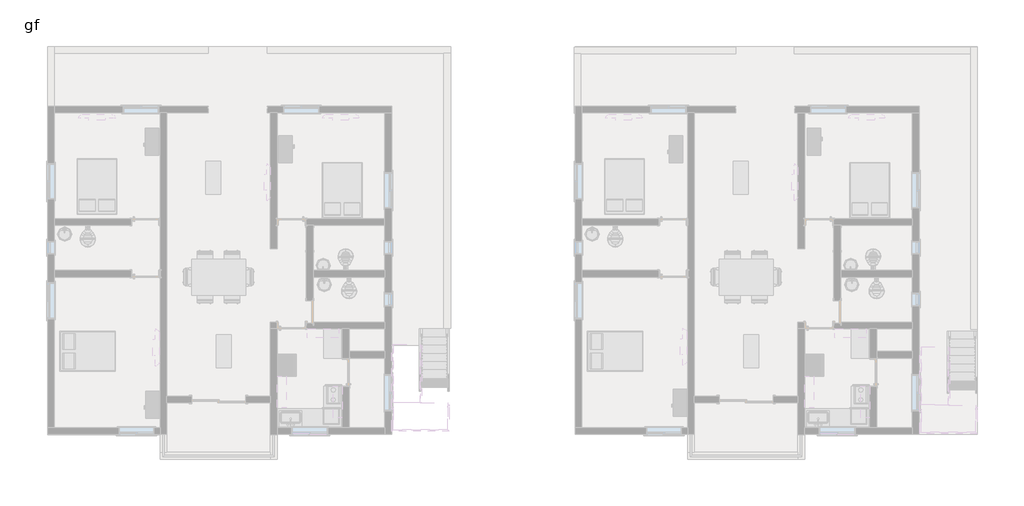
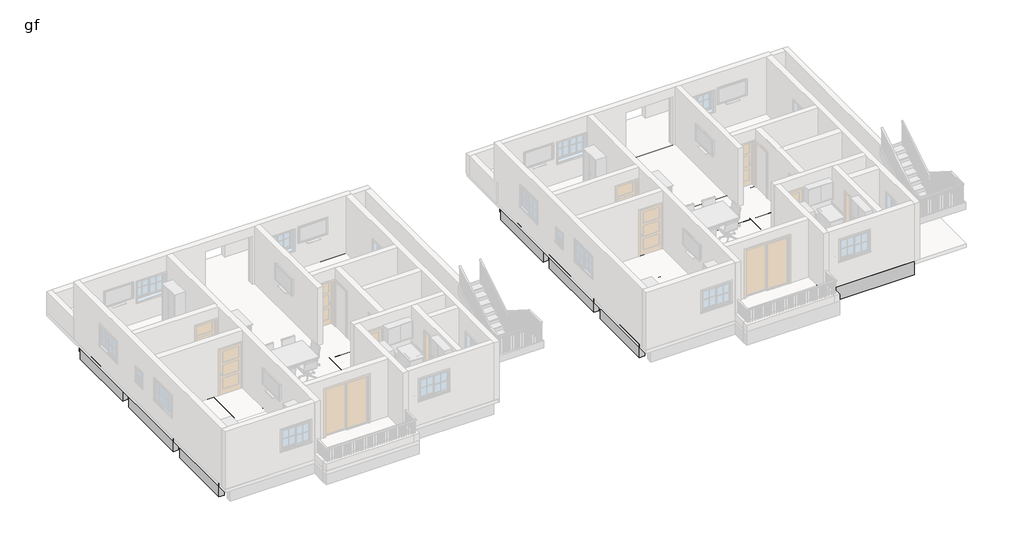
# One storey, part 3 of 8: 32 beams.
"""IFC4 building model written with IfcOpenShell, lengths in millimetres."""

from ifc_helpers import new_model, si_unit, origin, origin_with_axes, place, context, project, spatial, polyline, outline, extrude, faceted_brep, element, save

model = new_model("IFC4")

# Units and contexts
model_context = context("Model", 3, world=origin())
ifc_project = project(units=[si_unit("LENGTHUNIT", "METRE", prefix="MILLI")], contexts=[model_context])

# Site, building, storey
site = spatial("IfcSite", under=ifc_project)
building = spatial("IfcBuilding", under=site)
storey = spatial("IfcBuildingStorey", under=building, Name="gf", Elevation=609.6)

# Beams
placement = place(None, origin())
element("IfcBeam", 1, ObjectType="Concrete-Rectangular Beam", at=placement, inside=storey, context=model_context, shape_type="Brep", body=[
    faceted_brep([(-16071.9993763, -1252.5064015, 609.6), (-16300.5993763, -1252.5064015, 609.6), (-16300.5993763, -4148.1064015, 609.6), (-16071.9993763, -4148.1064015, 609.6), (-16300.5993763, -1252.5064015, 0.0), (-16300.5993763, -4148.1064015, 0.0), (-16071.9993763, -1252.5064015, 0.0), (-16071.9993763, -4148.1064015, 0.0)], [[[0, 1, 2, 3]], [[1, 4, 5, 2]], [[4, 6, 7, 5]], [[6, 0, 3, 7]], [[1, 0, 6, 4]], [[3, 2, 5, 7]]]),
    faceted_brep([(-16300.5993763, 6062.6935985, 609.6), (-16071.9993763, 6062.6935985, 609.6), (-16071.9993763, 6062.6935985, 0.0), (-16300.5993763, 6062.6935985, 0.0), (-16071.9993763, 2938.4935985, 609.6), (-16300.5993763, 2938.4935985, 609.6), (-16300.5993763, 2938.4935985, 0.0), (-16071.9993763, 2938.4935985, 0.0)], [[[0, 1, 2, 3]], [[4, 5, 6, 7]], [[1, 0, 5, 4]], [[0, 3, 6, 5]], [[3, 2, 7, 6]], [[2, 1, 4, 7]]]),
    faceted_brep([(-16300.5993763, 2481.2935985, 609.6), (-16071.9993763, 2481.2935985, 609.6), (-16071.9993763, 2481.2935985, 0.0), (-16300.5993763, 2481.2935985, 0.0), (-16071.9993763, -795.3064015, 609.6), (-16300.5993763, -795.3064015, 609.6), (-16300.5993763, -795.3064015, 0.0), (-16071.9993763, -795.3064015, 0.0), (-16071.9993763, 728.6935985, 609.6), (-16071.9993763, 957.2935985, 609.6), (-16071.9993763, 957.2935985, 0.0), (-16071.9993763, 728.6935985, 0.0)], [[[0, 1, 2, 3]], [[4, 5, 6, 7]], [[1, 0, 5, 4, 8, 9]], [[0, 3, 6, 5]], [[3, 2, 10, 11, 7, 6]], [[2, 1, 9, 8, 4, 7, 11, 10]]]),
])
element("IfcBeam", 2, ObjectType="Concrete-Rectangular Beam", at=placement, inside=storey, context=model_context, shape_type="SweptSolid", body=[
    extrude(outline(polyline([(-16071.9993763, 6291.2935985), (-16071.9993763, 6519.8935985), (-12490.5993763, 6519.8935985), (-12490.5993763, 6291.2935985), (-16071.9993763, 6291.2935985)])), origin_with_axes(), (0.0, 0.0, 1.0), 609.6),
    extrude(outline(polyline([(-12261.9993763, 6291.2935985), (-12261.9993763, 6519.8935985), (-8756.7993763, 6519.8935985), (-8756.7993763, 6291.2935985), (-12261.9993763, 6291.2935985)])), origin_with_axes(), (0.0, 0.0, 1.0), 609.6),
    extrude(outline(polyline([(-8528.1993763, 6291.2935985), (-8528.1993763, 6519.8935985), (-4870.5993763, 6519.8935985), (-4870.5993763, 6291.2935985), (-8528.1993763, 6291.2935985)])), origin_with_axes(), (0.0, 0.0, 1.0), 609.6),
])
element("IfcBeam", 3, ObjectType="Concrete-Rectangular Beam", at=placement, inside=storey, context=model_context, shape_type="Brep", body=[
    faceted_brep([(-12261.9993763, -1252.5064015, 609.6), (-12490.5993763, -1252.5064015, 609.6), (-12490.5993763, -4148.1064015, 609.6), (-12261.9993763, -4148.1064015, 609.6), (-12261.9993763, -3538.5064015, 609.6), (-12261.9993763, -3309.9064015, 609.6), (-12490.5993763, -1252.5064015, 0.0), (-12490.5993763, -4148.1064015, 0.0), (-12261.9993763, -1252.5064015, 0.0), (-12261.9993763, -3309.9064015, 0.0), (-12261.9993763, -3538.5064015, 0.0), (-12261.9993763, -4148.1064015, 0.0)], [[[0, 1, 2, 3, 4, 5]], [[1, 6, 7, 2]], [[6, 8, 9, 10, 11, 7]], [[8, 0, 5, 4, 3, 11, 10, 9]], [[1, 0, 8, 6]], [[3, 2, 7, 11]]]),
    faceted_brep([(-12490.5993763, 6062.6935985, 609.6), (-12261.9993763, 6062.6935985, 609.6), (-12261.9993763, 6062.6935985, 0.0), (-12490.5993763, 6062.6935985, 0.0), (-12261.9993763, 2938.4935985, 609.6), (-12490.5993763, 2938.4935985, 609.6), (-12490.5993763, 2938.4935985, 0.0), (-12261.9993763, 2938.4935985, 0.0)], [[[0, 1, 2, 3]], [[4, 5, 6, 7]], [[1, 0, 5, 4]], [[0, 3, 6, 5]], [[3, 2, 7, 6]], [[2, 1, 4, 7]]]),
    faceted_brep([(-12490.5993763, 2481.2935985, 609.6), (-12261.9993763, 2481.2935985, 609.6), (-12261.9993763, 2481.2935985, 0.0), (-12490.5993763, 2481.2935985, 0.0), (-12261.9993763, -795.3064015, 609.6), (-12490.5993763, -795.3064015, 609.6), (-12490.5993763, -795.3064015, 0.0), (-12261.9993763, -795.3064015, 0.0), (-12490.5993763, 957.2935985, 609.6), (-12490.5993763, 728.6935985, 609.6), (-12261.9993763, 728.6935985, 609.6), (-12261.9993763, 957.2935985, 609.6), (-12490.5993763, 957.2935985, 0.0), (-12490.5993763, 728.6935985, 0.0), (-12261.9993763, 957.2935985, 0.0), (-12261.9993763, 728.6935985, 0.0)], [[[0, 1, 2, 3]], [[4, 5, 6, 7]], [[1, 0, 8, 9, 5, 4, 10, 11]], [[0, 3, 12, 13, 6, 5, 9, 8]], [[3, 2, 14, 15, 7, 6, 13, 12]], [[2, 1, 11, 10, 4, 7, 15, 14]]]),
])
element("IfcBeam", 4, ObjectType="Concrete-Rectangular Beam", at=placement, inside=storey, context=model_context, shape_type="Brep", body=[
    faceted_brep([(-8528.1993763, 6062.6935985, 609.6), (-8756.7993763, 6062.6935985, 609.6), (-8756.7993763, 2938.4935985, 609.6), (-8528.1993763, 2938.4935985, 609.6), (-8528.1993763, 6062.6935985, 0.0), (-8528.1993763, 2938.4935985, 0.0), (-8756.7993763, 6062.6935985, 0.0), (-8756.7993763, 2938.4935985, 0.0)], [[[0, 1, 2, 3]], [[4, 0, 3, 5]], [[6, 4, 5, 7]], [[1, 6, 7, 2]], [[1, 0, 4, 6]], [[3, 2, 7, 5]]]),
    faceted_brep([(-8528.1993763, -5214.9064015, 609.6), (-8756.7993763, -5214.9064015, 609.6), (-8756.7993763, -5214.9064015, 0.0), (-8528.1993763, -5214.9064015, 0.0), (-8756.7993763, -4605.3064015, 609.6), (-8528.1993763, -4605.3064015, 609.6), (-8528.1993763, -4605.3064015, 0.0), (-8756.7993763, -4605.3064015, 0.0)], [[[0, 1, 2, 3]], [[4, 5, 6, 7]], [[1, 0, 5, 4]], [[0, 3, 6, 5]], [[3, 2, 7, 6]], [[2, 1, 4, 7]]]),
    faceted_brep([(-8528.1993763, -4148.1064015, 609.6), (-8756.7993763, -4148.1064015, 609.6), (-8756.7993763, -4148.1064015, 0.0), (-8528.1993763, -4148.1064015, 0.0), (-8756.7993763, -1252.5064015, 609.6), (-8528.1993763, -1252.5064015, 609.6), (-8528.1993763, -1252.5064015, 0.0), (-8756.7993763, -1252.5064015, 0.0), (-8756.7993763, -3309.9064015, 609.6), (-8756.7993763, -3538.5064015, 609.6), (-8756.7993763, -3538.5064015, 0.0), (-8756.7993763, -3309.9064015, 0.0)], [[[0, 1, 2, 3]], [[4, 5, 6, 7]], [[1, 0, 5, 4, 8, 9]], [[0, 3, 6, 5]], [[3, 2, 10, 11, 7, 6]], [[2, 1, 9, 8, 4, 7, 11, 10]]]),
    faceted_brep([(-8756.7993763, 2481.2935985, 609.6), (-8528.1993763, 2481.2935985, 609.6), (-8528.1993763, 2481.2935985, 0.0), (-8756.7993763, 2481.2935985, 0.0), (-8528.1993763, -795.3064015, 609.6), (-8756.7993763, -795.3064015, 609.6), (-8756.7993763, -795.3064015, 0.0), (-8528.1993763, -795.3064015, 0.0), (-8756.7993763, 957.2935985, 609.6), (-8756.7993763, 728.6935985, 609.6), (-8528.1993763, 728.6935985, 609.6), (-8528.1993763, 957.2935985, 609.6), (-8528.1993763, 728.6935985, 0.0), (-8528.1993763, 957.2935985, 0.0), (-8756.7993763, 728.6935985, 0.0), (-8756.7993763, 957.2935985, 0.0)], [[[0, 1, 2, 3]], [[4, 5, 6, 7]], [[1, 0, 8, 9, 5, 4, 10, 11]], [[2, 1, 11, 10, 4, 7, 12, 13]], [[3, 2, 13, 12, 7, 6, 14, 15]], [[0, 3, 15, 14, 6, 5, 9, 8]]]),
])
element("IfcBeam", 5, ObjectType="Concrete-Rectangular Beam", at=placement, inside=storey, context=model_context, shape_type="Brep", body=[
    faceted_brep([(-4641.9993763, -1023.9064015, 609.6), (-4870.5993763, -1023.9064015, 609.6), (-4870.5993763, -1785.9064015, 609.6), (-4870.5993763, -2014.5064015, 609.6), (-4870.5993763, -4148.1064015, 609.6), (-4641.9993763, -4148.1064015, 609.6), (-4870.5993763, -1023.9064015, 0.0), (-4870.5993763, -1785.9064015, 0.0), (-4870.5993763, -2014.5064015, 0.0), (-4870.5993763, -4148.1064015, 0.0), (-4641.9993763, -1023.9064015, 0.0), (-4641.9993763, -4148.1064015, 0.0)], [[[0, 1, 2, 3, 4, 5]], [[1, 6, 7, 8, 9, 4, 3, 2]], [[6, 10, 11, 9, 8, 7]], [[10, 0, 5, 11]], [[1, 0, 10, 6]], [[5, 4, 9, 11]]]),
    faceted_brep([(-4870.5993763, 6062.6935985, 609.6), (-4641.9993763, 6062.6935985, 609.6), (-4641.9993763, 6062.6935985, 0.0), (-4870.5993763, 6062.6935985, 0.0), (-4641.9993763, 2938.4935985, 609.6), (-4870.5993763, 2938.4935985, 609.6), (-4870.5993763, 2938.4935985, 0.0), (-4641.9993763, 2938.4935985, 0.0)], [[[0, 1, 2, 3]], [[4, 5, 6, 7]], [[1, 0, 5, 4]], [[0, 3, 6, 5]], [[3, 2, 7, 6]], [[2, 1, 4, 7]]]),
    faceted_brep([(-4870.5993763, 2481.2935985, 609.6), (-4641.9993763, 2481.2935985, 609.6), (-4641.9993763, 2481.2935985, 0.0), (-4870.5993763, 2481.2935985, 0.0), (-4641.9993763, -566.7064015, 609.6), (-4870.5993763, -566.7064015, 609.6), (-4870.5993763, -566.7064015, 0.0), (-4641.9993763, -566.7064015, 0.0), (-4870.5993763, 957.2935985, 609.6), (-4870.5993763, 728.6935985, 609.6), (-4870.5993763, 957.2935985, 0.0), (-4870.5993763, 728.6935985, 0.0)], [[[0, 1, 2, 3]], [[4, 5, 6, 7]], [[1, 0, 8, 9, 5, 4]], [[0, 3, 10, 11, 6, 5, 9, 8]], [[3, 2, 7, 6, 11, 10]], [[2, 1, 4, 7]]]),
])
element("IfcBeam", 6, ObjectType="Concrete-Rectangular Beam", at=placement, inside=storey, context=model_context, shape_type="Brep", body=[
    faceted_brep([(-7308.9993763, 2709.8935985, 609.6), (-7537.5993763, 2709.8935985, 609.6), (-7537.5993763, 2481.2935985, 609.6), (-7537.5993763, 957.2935985, 609.6), (-7537.5993763, 728.6935985, 609.6), (-7537.5993763, -795.3064015, 609.6), (-7308.9993763, -795.3064015, 609.6), (-7308.9993763, 728.6935985, 609.6), (-7308.9993763, 957.2935985, 609.6), (-7308.9993763, 2481.2935985, 609.6), (-7308.9993763, 2709.8935985, 0.0), (-7308.9993763, -795.3064015, 0.0), (-7308.9993763, 728.6935985, 0.0), (-7308.9993763, 957.2935985, 0.0), (-7308.9993763, 2481.2935985, 0.0), (-7537.5993763, 2709.8935985, 0.0), (-7537.5993763, -795.3064015, 0.0), (-7537.5993763, 728.6935985, 0.0), (-7537.5993763, 957.2935985, 0.0), (-7537.5993763, 2481.2935985, 0.0)], [[[0, 1, 2, 3, 4, 5, 6, 7, 8, 9]], [[10, 0, 9, 8, 7, 6, 11, 12, 13, 14]], [[15, 10, 14, 13, 12, 11, 16, 17, 18, 19]], [[1, 15, 19, 18, 17, 16, 5, 4, 3, 2]], [[6, 5, 16, 11]], [[1, 0, 10, 15]]]),
])
element("IfcBeam", 7, ObjectType="Concrete-Rectangular Beam", at=placement, inside=storey, context=model_context, shape_type="SweptSolid", body=[
    extrude(outline(polyline([(-7308.9993763, 2481.2935985), (-7308.9993763, 2709.8935985), (-4870.5993763, 2709.8935985), (-4870.5993763, 2481.2935985), (-7308.9993763, 2481.2935985)])), origin_with_axes(), (0.0, 0.0, 1.0), 609.6),
])
element("IfcBeam", 8, ObjectType="Concrete-Rectangular Beam", at=placement, inside=storey, context=model_context, shape_type="SweptSolid", body=[
    extrude(outline(polyline([(-4870.5993763, 957.2935985), (-4870.5993763, 728.6935985), (-7308.9993763, 728.6935985), (-7308.9993763, 957.2935985), (-4870.5993763, 957.2935985)])), origin_with_axes(), (0.0, 0.0, 1.0), 609.6),
])
element("IfcBeam", 9, ObjectType="Concrete-Rectangular Beam", at=placement, inside=storey, context=model_context, shape_type="SweptSolid", body=[
    extrude(outline(polyline([(-12261.9993763, 2481.2935985), (-12261.9993763, 2709.8935985), (-8756.7993763, 2709.8935985), (-8756.7993763, 2481.2935985), (-12261.9993763, 2481.2935985)])), origin_with_axes(), (0.0, 0.0, 1.0), 609.6),
    extrude(outline(polyline([(-7537.5993763, 2709.8935985), (-7537.5993763, 2481.2935985), (-8528.1993763, 2481.2935985), (-8528.1993763, 2709.8935985), (-7537.5993763, 2709.8935985)])), origin_with_axes(), (0.0, 0.0, 1.0), 609.6),
])
element("IfcBeam", 10, ObjectType="Concrete-Rectangular Beam", at=placement, inside=storey, context=model_context, shape_type="Brep", body=[
    faceted_brep([(-13481.1993763, 2709.8935985, 609.6), (-13709.7993763, 2709.8935985, 609.6), (-13709.7993763, 957.2935985, 609.6), (-13709.7993763, 728.6935985, 609.6), (-13709.7993763, -795.3064015, 609.6), (-13481.1993763, -795.3064015, 609.6), (-13481.1993763, 728.6935985, 609.6), (-13481.1993763, 957.2935985, 609.6), (-13481.1993763, 2481.2935985, 609.6), (-13709.7993763, 2709.8935985, 0.0), (-13709.7993763, 957.2935985, 0.0), (-13709.7993763, 728.6935985, 0.0), (-13709.7993763, -795.3064015, 0.0), (-13481.1993763, 2709.8935985, 0.0), (-13481.1993763, 2481.2935985, 0.0), (-13481.1993763, 957.2935985, 0.0), (-13481.1993763, 728.6935985, 0.0), (-13481.1993763, -795.3064015, 0.0)], [[[0, 1, 2, 3, 4, 5, 6, 7, 8]], [[1, 9, 10, 11, 12, 4, 3, 2]], [[9, 13, 14, 15, 16, 17, 12, 11, 10]], [[13, 0, 8, 7, 6, 5, 17, 16, 15, 14]], [[5, 4, 12, 17]], [[1, 0, 13, 9]]]),
])
element("IfcBeam", 11, ObjectType="Concrete-Rectangular Beam", at=placement, inside=storey, context=model_context, shape_type="SweptSolid", body=[
    extrude(outline(polyline([(-16071.9993763, 728.6935985), (-16071.9993763, 957.2935985), (-13709.7993763, 957.2935985), (-13709.7993763, 728.6935985), (-16071.9993763, 728.6935985)])), origin_with_axes(), (0.0, 0.0, 1.0), 609.6),
])
element("IfcBeam", 12, ObjectType="Concrete-Rectangular Beam", at=placement, inside=storey, context=model_context, shape_type="SweptSolid", body=[
    extrude(outline(polyline([(-12490.5993763, 957.2935985), (-12490.5993763, 728.6935985), (-13481.1993763, 728.6935985), (-13481.1993763, 957.2935985), (-12490.5993763, 957.2935985)])), origin_with_axes(), (0.0, 0.0, 1.0), 609.6),
])
element("IfcBeam", 13, ObjectType="Concrete-Rectangular Beam", at=placement, inside=storey, context=model_context, shape_type="SweptSolid", body=[
    extrude(outline(polyline([(-12261.9993763, 728.6935985), (-12261.9993763, 957.2935985), (-8756.7993763, 957.2935985), (-8756.7993763, 728.6935985), (-12261.9993763, 728.6935985)])), origin_with_axes(), (0.0, 0.0, 1.0), 609.6),
    extrude(outline(polyline([(-7537.5993763, 957.2935985), (-7537.5993763, 728.6935985), (-8528.1993763, 728.6935985), (-8528.1993763, 957.2935985), (-7537.5993763, 957.2935985)])), origin_with_axes(), (0.0, 0.0, 1.0), 609.6),
])
element("IfcBeam", 14, ObjectType="Concrete-Rectangular Beam", at=placement, inside=storey, context=model_context, shape_type="SweptSolid", body=[
    extrude(outline(polyline([(-12490.5993763, 2709.8935985), (-12490.5993763, 2481.2935985), (-13481.1993763, 2481.2935985), (-13481.1993763, 2709.8935985), (-12490.5993763, 2709.8935985)])), origin_with_axes(), (0.0, 0.0, 1.0), 609.6),
])
element("IfcBeam", 15, ObjectType="Concrete-Rectangular Beam", at=placement, inside=storey, context=model_context, shape_type="Brep", body=[
    faceted_brep([(1802.5761273, -1252.5064015, 609.6), (1573.9761273, -1252.5064015, 609.6), (1573.9761273, -4148.1064015, 609.6), (1802.5761273, -4148.1064015, 609.6), (1573.9761273, -1252.5064015, 0.0), (1573.9761273, -4148.1064015, 0.0), (1802.5761273, -1252.5064015, 0.0), (1802.5761273, -4148.1064015, 0.0)], [[[0, 1, 2, 3]], [[1, 4, 5, 2]], [[4, 6, 7, 5]], [[6, 0, 3, 7]], [[1, 0, 6, 4]], [[3, 2, 5, 7]]]),
    faceted_brep([(1573.9761273, 6062.6935985, 609.6), (1802.5761273, 6062.6935985, 609.6), (1802.5761273, 6062.6935985, 0.0), (1573.9761273, 6062.6935985, 0.0), (1802.5761273, 2938.4935985, 609.6), (1573.9761273, 2938.4935985, 609.6), (1573.9761273, 2938.4935985, 0.0), (1802.5761273, 2938.4935985, 0.0)], [[[0, 1, 2, 3]], [[4, 5, 6, 7]], [[1, 0, 5, 4]], [[0, 3, 6, 5]], [[3, 2, 7, 6]], [[2, 1, 4, 7]]]),
    faceted_brep([(1573.9761273, 2481.2935985, 609.6), (1802.5761273, 2481.2935985, 609.6), (1802.5761273, 2481.2935985, 0.0), (1573.9761273, 2481.2935985, 0.0), (1802.5761273, -795.3064015, 609.6), (1573.9761273, -795.3064015, 609.6), (1573.9761273, -795.3064015, 0.0), (1802.5761273, -795.3064015, 0.0), (1802.5761273, 728.6935985, 609.6), (1802.5761273, 957.2935985, 609.6), (1802.5761273, 957.2935985, 0.0), (1802.5761273, 728.6935985, 0.0)], [[[0, 1, 2, 3]], [[4, 5, 6, 7]], [[1, 0, 5, 4, 8, 9]], [[0, 3, 6, 5]], [[3, 2, 10, 11, 7, 6]], [[2, 1, 9, 8, 4, 7, 11, 10]]]),
])
element("IfcBeam", 16, ObjectType="Concrete-Rectangular Beam", at=placement, inside=storey, context=model_context, shape_type="SweptSolid", body=[
    extrude(outline(polyline([(1802.5761273, 6291.2935985), (1802.5761273, 6519.8935985), (5383.9761273, 6519.8935985), (5383.9761273, 6291.2935985), (1802.5761273, 6291.2935985)])), origin_with_axes(), (0.0, 0.0, 1.0), 609.6),
    extrude(outline(polyline([(5612.5761273, 6291.2935985), (5612.5761273, 6519.8935985), (9117.7761273, 6519.8935985), (9117.7761273, 6291.2935985), (5612.5761273, 6291.2935985)])), origin_with_axes(), (0.0, 0.0, 1.0), 609.6),
    extrude(outline(polyline([(9346.3761273, 6291.2935985), (9346.3761273, 6519.8935985), (13003.9761273, 6519.8935985), (13003.9761273, 6291.2935985), (9346.3761273, 6291.2935985)])), origin_with_axes(), (0.0, 0.0, 1.0), 609.6),
])
element("IfcBeam", 17, ObjectType="Concrete-Rectangular Beam", at=placement, inside=storey, context=model_context, shape_type="Brep", body=[
    faceted_brep([(5612.5761273, -1252.5064015, 609.6), (5383.9761273, -1252.5064015, 609.6), (5383.9761273, -4148.1064015, 609.6), (5612.5761273, -4148.1064015, 609.6), (5612.5761273, -3538.5064015, 609.6), (5612.5761273, -3309.9064015, 609.6), (5383.9761273, -1252.5064015, 0.0), (5383.9761273, -4148.1064015, 0.0), (5612.5761273, -1252.5064015, 0.0), (5612.5761273, -3309.9064015, 0.0), (5612.5761273, -3538.5064015, 0.0), (5612.5761273, -4148.1064015, 0.0)], [[[0, 1, 2, 3, 4, 5]], [[1, 6, 7, 2]], [[6, 8, 9, 10, 11, 7]], [[8, 0, 5, 4, 3, 11, 10, 9]], [[1, 0, 8, 6]], [[3, 2, 7, 11]]]),
    faceted_brep([(5383.9761273, 6062.6935985, 609.6), (5612.5761273, 6062.6935985, 609.6), (5612.5761273, 6062.6935985, 0.0), (5383.9761273, 6062.6935985, 0.0), (5612.5761273, 2938.4935985, 609.6), (5383.9761273, 2938.4935985, 609.6), (5383.9761273, 2938.4935985, 0.0), (5612.5761273, 2938.4935985, 0.0)], [[[0, 1, 2, 3]], [[4, 5, 6, 7]], [[1, 0, 5, 4]], [[0, 3, 6, 5]], [[3, 2, 7, 6]], [[2, 1, 4, 7]]]),
    faceted_brep([(5383.9761273, 2481.2935985, 609.6), (5612.5761273, 2481.2935985, 609.6), (5612.5761273, 2481.2935985, 0.0), (5383.9761273, 2481.2935985, 0.0), (5612.5761273, -795.3064015, 609.6), (5383.9761273, -795.3064015, 609.6), (5383.9761273, -795.3064015, 0.0), (5612.5761273, -795.3064015, 0.0), (5383.9761273, 957.2935985, 609.6), (5383.9761273, 728.6935985, 609.6), (5612.5761273, 728.6935985, 609.6), (5612.5761273, 957.2935985, 609.6), (5383.9761273, 957.2935985, 0.0), (5383.9761273, 728.6935985, 0.0), (5612.5761273, 957.2935985, 0.0), (5612.5761273, 728.6935985, 0.0)], [[[0, 1, 2, 3]], [[4, 5, 6, 7]], [[1, 0, 8, 9, 5, 4, 10, 11]], [[0, 3, 12, 13, 6, 5, 9, 8]], [[3, 2, 14, 15, 7, 6, 13, 12]], [[2, 1, 11, 10, 4, 7, 15, 14]]]),
])
element("IfcBeam", 18, ObjectType="Concrete-Rectangular Beam", at=placement, inside=storey, context=model_context, shape_type="Brep", body=[
    faceted_brep([(9346.3761273, 6062.6935985, 609.6), (9117.7761273, 6062.6935985, 609.6), (9117.7761273, 2938.4935985, 609.6), (9346.3761273, 2938.4935985, 609.6), (9346.3761273, 6062.6935985, 0.0), (9346.3761273, 2938.4935985, 0.0), (9117.7761273, 6062.6935985, 0.0), (9117.7761273, 2938.4935985, 0.0)], [[[0, 1, 2, 3]], [[4, 0, 3, 5]], [[6, 4, 5, 7]], [[1, 6, 7, 2]], [[1, 0, 4, 6]], [[3, 2, 7, 5]]]),
    faceted_brep([(9346.3761273, -5214.9064015, 609.6), (9117.7761273, -5214.9064015, 609.6), (9117.7761273, -5214.9064015, 0.0), (9346.3761273, -5214.9064015, 0.0), (9117.7761273, -4605.3064015, 609.6), (9346.3761273, -4605.3064015, 609.6), (9346.3761273, -4605.3064015, 0.0), (9117.7761273, -4605.3064015, 0.0)], [[[0, 1, 2, 3]], [[4, 5, 6, 7]], [[1, 0, 5, 4]], [[6, 5, 0, 3]], [[3, 2, 7, 6]], [[2, 1, 4, 7]]]),
    faceted_brep([(9346.3761273, -4148.1064015, 609.6), (9117.7761273, -4148.1064015, 609.6), (9117.7761273, -4148.1064015, 0.0), (9346.3761273, -4148.1064015, 0.0), (9117.7761273, -1252.5064015, 609.6), (9346.3761273, -1252.5064015, 609.6), (9346.3761273, -1252.5064015, 0.0), (9117.7761273, -1252.5064015, 0.0), (9117.7761273, -3309.9064015, 609.6), (9117.7761273, -3538.5064015, 609.6), (9117.7761273, -3538.5064015, 0.0), (9117.7761273, -3309.9064015, 0.0)], [[[0, 1, 2, 3]], [[4, 5, 6, 7]], [[1, 0, 5, 4, 8, 9]], [[0, 3, 6, 5]], [[3, 2, 10, 11, 7, 6]], [[2, 1, 9, 8, 4, 7, 11, 10]]]),
    faceted_brep([(9117.7761273, 2481.2935985, 609.6), (9346.3761273, 2481.2935985, 609.6), (9346.3761273, 2481.2935985, 0.0), (9117.7761273, 2481.2935985, 0.0), (9346.3761273, -795.3064015, 609.6), (9117.7761273, -795.3064015, 609.6), (9117.7761273, -795.3064015, 0.0), (9346.3761273, -795.3064015, 0.0), (9117.7761273, 957.2935985, 609.6), (9117.7761273, 728.6935985, 609.6), (9346.3761273, 728.6935985, 609.6), (9346.3761273, 957.2935985, 609.6), (9346.3761273, 728.6935985, 0.0), (9346.3761273, 957.2935985, 0.0), (9117.7761273, 728.6935985, 0.0), (9117.7761273, 957.2935985, 0.0)], [[[0, 1, 2, 3]], [[4, 5, 6, 7]], [[1, 0, 8, 9, 5, 4, 10, 11]], [[2, 1, 11, 10, 4, 7, 12, 13]], [[3, 2, 13, 12, 7, 6, 14, 15]], [[0, 3, 15, 14, 6, 5, 9, 8]]]),
])
element("IfcBeam", 19, ObjectType="Concrete-Rectangular Beam", at=placement, inside=storey, context=model_context, shape_type="Brep", body=[
    faceted_brep([(9346.3761273, -4376.7064015, 609.6), (9346.3761273, -4605.3064015, 609.6), (13003.9761273, -4605.3064015, 609.6), (13003.9761273, -4376.7064015, 609.6), (11784.7761273, -4376.7064015, 609.6), (11556.1761273, -4376.7064015, 609.6), (9346.3761273, -4376.7064015, 0.0), (13003.9761273, -4376.7064015, 0.0), (11784.7761273, -4376.7064015, 0.0), (11556.1761273, -4376.7064015, 0.0), (9346.3761273, -4605.3064015, 0.0), (13003.9761273, -4605.3064015, 0.0)], [[[0, 1, 2, 3, 4, 5]], [[6, 0, 5, 4, 3, 7, 8, 9]], [[10, 6, 9, 8, 7, 11]], [[1, 10, 11, 2]], [[1, 0, 6, 10]], [[3, 2, 11, 7]]]),
])
element("IfcBeam", 20, ObjectType="Concrete-Rectangular Beam", at=placement, inside=storey, context=model_context, shape_type="Brep", body=[
    faceted_brep([(13232.5761273, -1023.9064015, 609.6), (13003.9761273, -1023.9064015, 609.6), (13003.9761273, -1785.9064015, 609.6), (13003.9761273, -2014.5064015, 609.6), (13003.9761273, -4148.1064015, 609.6), (13232.5761273, -4148.1064015, 609.6), (13003.9761273, -1023.9064015, 0.0), (13003.9761273, -1785.9064015, 0.0), (13003.9761273, -2014.5064015, 0.0), (13003.9761273, -4148.1064015, 0.0), (13232.5761273, -1023.9064015, 0.0), (13232.5761273, -4148.1064015, 0.0)], [[[0, 1, 2, 3, 4, 5]], [[1, 6, 7, 8, 9, 4, 3, 2]], [[6, 10, 11, 9, 8, 7]], [[10, 0, 5, 11]], [[1, 0, 10, 6]], [[5, 4, 9, 11]]]),
    faceted_brep([(13003.9761273, 6062.6935985, 609.6), (13232.5761273, 6062.6935985, 609.6), (13232.5761273, 6062.6935985, 0.0), (13003.9761273, 6062.6935985, 0.0), (13232.5761273, 2938.4935985, 609.6), (13003.9761273, 2938.4935985, 609.6), (13003.9761273, 2938.4935985, 0.0), (13232.5761273, 2938.4935985, 0.0)], [[[0, 1, 2, 3]], [[4, 5, 6, 7]], [[1, 0, 5, 4]], [[0, 3, 6, 5]], [[3, 2, 7, 6]], [[2, 1, 4, 7]]]),
    faceted_brep([(13003.9761273, 2481.2935985, 609.6), (13232.5761273, 2481.2935985, 609.6), (13232.5761273, 2481.2935985, 0.0), (13003.9761273, 2481.2935985, 0.0), (13232.5761273, -566.7064015, 609.6), (13003.9761273, -566.7064015, 609.6), (13003.9761273, -566.7064015, 0.0), (13232.5761273, -566.7064015, 0.0), (13003.9761273, 957.2935985, 609.6), (13003.9761273, 728.6935985, 609.6), (13003.9761273, 957.2935985, 0.0), (13003.9761273, 728.6935985, 0.0)], [[[0, 1, 2, 3]], [[4, 5, 6, 7]], [[1, 0, 8, 9, 5, 4]], [[0, 3, 10, 11, 6, 5, 9, 8]], [[3, 2, 7, 6, 11, 10]], [[2, 1, 4, 7]]]),
])
element("IfcBeam", 21, ObjectType="Concrete-Rectangular Beam", at=placement, inside=storey, context=model_context, shape_type="Brep", body=[
    faceted_brep([(9346.3761273, -795.3064015, 609.6), (9346.3761273, -1023.9064015, 609.6), (11556.1761273, -1023.9064015, 609.6), (11784.7761273, -1023.9064015, 609.6), (13003.9761273, -1023.9064015, 609.6), (13003.9761273, -795.3064015, 609.6), (10565.5761273, -795.3064015, 609.6), (10336.9761273, -795.3064015, 609.6), (9346.3761273, -795.3064015, 0.0), (13003.9761273, -795.3064015, 0.0), (10565.5761273, -795.3064015, 0.0), (10336.9761273, -795.3064015, 0.0), (9346.3761273, -1023.9064015, 0.0), (13003.9761273, -1023.9064015, 0.0), (11784.7761273, -1023.9064015, 0.0), (11556.1761273, -1023.9064015, 0.0)], [[[0, 1, 2, 3, 4, 5, 6, 7]], [[8, 0, 7, 6, 5, 9, 10, 11]], [[12, 8, 11, 10, 9, 13, 14, 15]], [[1, 12, 15, 14, 13, 4, 3, 2]], [[1, 0, 8, 12]], [[5, 4, 13, 9]]]),
])
element("IfcBeam", 22, ObjectType="Concrete-Rectangular Beam", at=placement, inside=storey, context=model_context, shape_type="Brep", body=[
    faceted_brep([(11556.1761273, -4376.7064015, 609.6), (11784.7761273, -4376.7064015, 609.6), (11784.7761273, -2014.5064015, 609.6), (11784.7761273, -1785.9064015, 609.6), (11784.7761273, -1023.9064015, 609.6), (11556.1761273, -1023.9064015, 609.6), (11784.7761273, -4376.7064015, 0.0), (11784.7761273, -2014.5064015, 0.0), (11784.7761273, -1785.9064015, 0.0), (11784.7761273, -1023.9064015, 0.0), (11556.1761273, -4376.7064015, 0.0), (11556.1761273, -1023.9064015, 0.0)], [[[0, 1, 2, 3, 4, 5]], [[1, 6, 7, 8, 9, 4, 3, 2]], [[6, 10, 11, 9, 8, 7]], [[10, 0, 5, 11]], [[1, 0, 10, 6]], [[5, 4, 9, 11]]]),
])
element("IfcBeam", 23, ObjectType="Concrete-Rectangular Beam", at=placement, inside=storey, context=model_context, shape_type="SweptSolid", body=[
    extrude(outline(polyline([(13003.9761273, -1785.9064015), (13003.9761273, -2014.5064015), (11784.7761273, -2014.5064015), (11784.7761273, -1785.9064015), (13003.9761273, -1785.9064015)])), origin_with_axes(), (0.0, 0.0, 1.0), 609.6),
])
element("IfcBeam", 24, ObjectType="Concrete-Rectangular Beam", at=placement, inside=storey, context=model_context, shape_type="Brep", body=[
    faceted_brep([(10565.5761273, 2709.8935985, 609.6), (10336.9761273, 2709.8935985, 609.6), (10336.9761273, 2481.2935985, 609.6), (10336.9761273, 957.2935985, 609.6), (10336.9761273, 728.6935985, 609.6), (10336.9761273, -795.3064015, 609.6), (10565.5761273, -795.3064015, 609.6), (10565.5761273, 728.6935985, 609.6), (10565.5761273, 957.2935985, 609.6), (10565.5761273, 2481.2935985, 609.6), (10565.5761273, 2709.8935985, 0.0), (10565.5761273, -795.3064015, 0.0), (10565.5761273, 728.6935985, 0.0), (10565.5761273, 957.2935985, 0.0), (10565.5761273, 2481.2935985, 0.0), (10336.9761273, 2709.8935985, 0.0), (10336.9761273, -795.3064015, 0.0), (10336.9761273, 728.6935985, 0.0), (10336.9761273, 957.2935985, 0.0), (10336.9761273, 2481.2935985, 0.0)], [[[0, 1, 2, 3, 4, 5, 6, 7, 8, 9]], [[10, 0, 9, 8, 7, 6, 11, 12, 13, 14]], [[15, 10, 14, 13, 12, 11, 16, 17, 18, 19]], [[1, 15, 19, 18, 17, 16, 5, 4, 3, 2]], [[6, 5, 16, 11]], [[1, 0, 10, 15]]]),
])
element("IfcBeam", 25, ObjectType="Concrete-Rectangular Beam", at=placement, inside=storey, context=model_context, shape_type="SweptSolid", body=[
    extrude(outline(polyline([(10565.5761273, 2481.2935985), (10565.5761273, 2709.8935985), (13003.9761273, 2709.8935985), (13003.9761273, 2481.2935985), (10565.5761273, 2481.2935985)])), origin_with_axes(), (0.0, 0.0, 1.0), 609.6),
])
element("IfcBeam", 26, ObjectType="Concrete-Rectangular Beam", at=placement, inside=storey, context=model_context, shape_type="SweptSolid", body=[
    extrude(outline(polyline([(13003.9761273, 957.2935985), (13003.9761273, 728.6935985), (10565.5761273, 728.6935985), (10565.5761273, 957.2935985), (13003.9761273, 957.2935985)])), origin_with_axes(), (0.0, 0.0, 1.0), 609.6),
])
element("IfcBeam", 27, ObjectType="Concrete-Rectangular Beam", at=placement, inside=storey, context=model_context, shape_type="SweptSolid", body=[
    extrude(outline(polyline([(5612.5761273, 2481.2935985), (5612.5761273, 2709.8935985), (9117.7761273, 2709.8935985), (9117.7761273, 2481.2935985), (5612.5761273, 2481.2935985)])), origin_with_axes(), (0.0, 0.0, 1.0), 609.6),
    extrude(outline(polyline([(10336.9761273, 2709.8935985), (10336.9761273, 2481.2935985), (9346.3761273, 2481.2935985), (9346.3761273, 2709.8935985), (10336.9761273, 2709.8935985)])), origin_with_axes(), (0.0, 0.0, 1.0), 609.6),
])
element("IfcBeam", 28, ObjectType="Concrete-Rectangular Beam", at=placement, inside=storey, context=model_context, shape_type="Brep", body=[
    faceted_brep([(4393.3761273, 2709.8935985, 609.6), (4164.7761273, 2709.8935985, 609.6), (4164.7761273, 957.2935985, 609.6), (4164.7761273, 728.6935985, 609.6), (4164.7761273, -795.3064015, 609.6), (4393.3761273, -795.3064015, 609.6), (4393.3761273, 728.6935985, 609.6), (4393.3761273, 957.2935985, 609.6), (4393.3761273, 2481.2935985, 609.6), (4164.7761273, 2709.8935985, 0.0), (4164.7761273, 957.2935985, 0.0), (4164.7761273, 728.6935985, 0.0), (4164.7761273, -795.3064015, 0.0), (4393.3761273, 2709.8935985, 0.0), (4393.3761273, 2481.2935985, 0.0), (4393.3761273, 957.2935985, 0.0), (4393.3761273, 728.6935985, 0.0), (4393.3761273, -795.3064015, 0.0)], [[[0, 1, 2, 3, 4, 5, 6, 7, 8]], [[1, 9, 10, 11, 12, 4, 3, 2]], [[9, 13, 14, 15, 16, 17, 12, 11, 10]], [[13, 0, 8, 7, 6, 5, 17, 16, 15, 14]], [[5, 4, 12, 17]], [[1, 0, 13, 9]]]),
])
element("IfcBeam", 29, ObjectType="Concrete-Rectangular Beam", at=placement, inside=storey, context=model_context, shape_type="SweptSolid", body=[
    extrude(outline(polyline([(1802.5761273, 728.6935985), (1802.5761273, 957.2935985), (4164.7761273, 957.2935985), (4164.7761273, 728.6935985), (1802.5761273, 728.6935985)])), origin_with_axes(), (0.0, 0.0, 1.0), 609.6),
])
element("IfcBeam", 30, ObjectType="Concrete-Rectangular Beam", at=placement, inside=storey, context=model_context, shape_type="SweptSolid", body=[
    extrude(outline(polyline([(5383.9761273, 957.2935985), (5383.9761273, 728.6935985), (4393.3761273, 728.6935985), (4393.3761273, 957.2935985), (5383.9761273, 957.2935985)])), origin_with_axes(), (0.0, 0.0, 1.0), 609.6),
])
element("IfcBeam", 31, ObjectType="Concrete-Rectangular Beam", at=placement, inside=storey, context=model_context, shape_type="SweptSolid", body=[
    extrude(outline(polyline([(5612.5761273, 728.6935985), (5612.5761273, 957.2935985), (9117.7761273, 957.2935985), (9117.7761273, 728.6935985), (5612.5761273, 728.6935985)])), origin_with_axes(), (0.0, 0.0, 1.0), 609.6),
    extrude(outline(polyline([(10336.9761273, 957.2935985), (10336.9761273, 728.6935985), (9346.3761273, 728.6935985), (9346.3761273, 957.2935985), (10336.9761273, 957.2935985)])), origin_with_axes(), (0.0, 0.0, 1.0), 609.6),
])
element("IfcBeam", 32, ObjectType="Concrete-Rectangular Beam", at=placement, inside=storey, context=model_context, shape_type="SweptSolid", body=[
    extrude(outline(polyline([(5383.9761273, 2709.8935985), (5383.9761273, 2481.2935985), (4393.3761273, 2481.2935985), (4393.3761273, 2709.8935985), (5383.9761273, 2709.8935985)])), origin_with_axes(), (0.0, 0.0, 1.0), 609.6),
])

save(model, "model.ifc")

# Revit data of these elements
# Type "Concrete-Rectangular Beam"
#   Assembly Code = "B10"
#   Length [instance default] = 5' - 0"
#   b = 0' - 9"
#   h = 2' - 0"
#   Structural Material [instance default] = Concrete, Cast-in-Place gray
# Elements 1, 2, 3, 4, 5, 6, 7, 8, 9, 10, 11, 12, 13, 14, 15, 16, 17, 18, 19, 20, 21, 22, 23, 24, 25, 26, 27, 28, 29, 30, 31, 32 (IfcBeam, "Concrete-Rectangular Beam")
#   Structural Material = Concrete, Cast-in-Place gray
#   Phase Created = New Construction
#   Materials on its faces: "Concrete, Cast-in-Place gray"
# Materials
#   "Concrete, Cast-in-Place gray": class "Concrete", colour RGB 192 192 192, transparency 0, Description = "Cast-in-place concrete", Cost = 0
